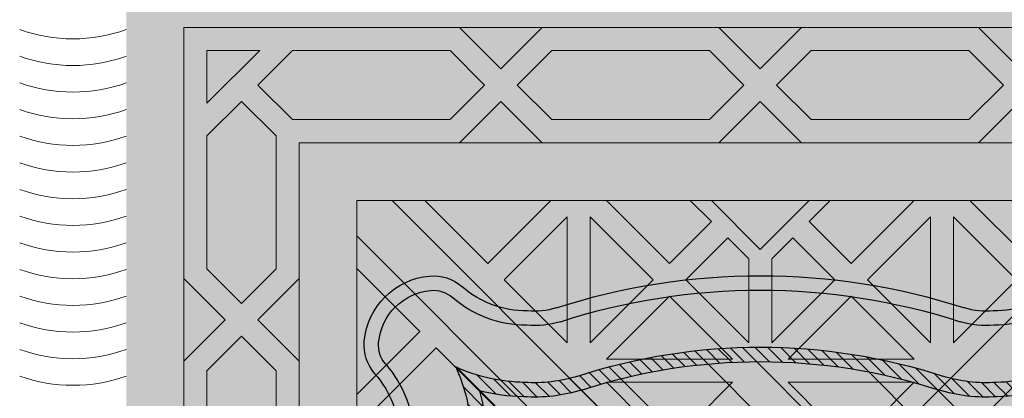
# Model space of a CAD drawing. Units: inches. Extents: x 844 to 2234, y 346 to 1084.
# Tile 33 of 93: x 1249.18 to 1260.07, y 703.6 to 707.78. Entities that reach past the tile are written whole.
import ezdxf

# ---------------------------------------------------------------- set-up
doc = ezdxf.new("R2010")
doc.units = ezdxf.units.IN
doc.header["$MEASUREMENT"] = 0
doc.layers.add('furniture', color=8, linetype='Continuous', lineweight=18)
doc.layers.add('RA-AP-01$0$INT', color=35, linetype='Continuous', lineweight=5)
doc.layers.add('RA-AP-01$0$FURN', color=3, linetype='Continuous')
doc.layers.add('RA-AP-01$0$WOOD', color=64, linetype='Continuous')

# ---------------------------------------------------------------- blocks, each defined once
blk = doc.blocks.new('A$C18D01794')
at = {"layer": 'RA-AP-01$0$INT'}
h = blk.add_hatch(color=256, dxfattribs=at)
h.paths.add_polyline_path([(4.35521, -6.15671), (4.35521, -8.05671), (5.45521, -8.05671), (5.45521, -6.15671)])
h.paths.add_polyline_path([(4.40521, -8.00671), (4.40521, -6.20671), (5.40521, -6.20671), (5.40521, -8.00671)], flags=16)
h = blk.add_hatch(color=256, dxfattribs=at)
h.paths.add_polyline_path([(4.50521, -7.5855), (4.46935, -7.54964), (4.50521, -7.51378), (4.50521, -7.38196), (4.46935, -7.34611), (4.50521, -7.31025), (4.50521, -7.17843), (4.46935, -7.14257), (4.50521, -7.10671), (4.47692, -7.10671), (4.45521, -7.12843), (4.43349, -7.10671), (4.40521, -7.10671), (4.44106, -7.14257), (4.40521, -7.17843), (4.40521, -7.31025), (4.44106, -7.34611), (4.40521, -7.38196), (4.40521, -7.51378), (4.44106, -7.54964), (4.40521, -7.5855), (4.40521, -7.71732), (4.44106, -7.75318), (4.40521, -7.78903), (4.40521, -8.00671), (4.64435, -8.00671), (4.68021, -7.97085), (4.71606, -8.00671), (4.86935, -8.00671), (4.90521, -7.97085), (4.94106, -8.00671), (5.09435, -8.00671), (5.13021, -7.97085), (5.16606, -8.00671), (5.40521, -8.00671), (5.40521, -7.78903), (5.36935, -7.75318), (5.40521, -7.71732), (5.40521, -7.5855), (5.36935, -7.54964), (5.40521, -7.51378), (5.40521, -7.38196), (5.36935, -7.34611), (5.40521, -7.31025), (5.40521, -7.17843), (5.36935, -7.14257), (5.40521, -7.10671), (5.37692, -7.10671), (5.35521, -7.12843), (5.33349, -7.10671), (5.30521, -7.10671), (5.34106, -7.14257), (5.30521, -7.17843), (5.30521, -7.31025), (5.34106, -7.34611), (5.30521, -7.38196), (5.30521, -7.51378), (5.34106, -7.54964), (5.30521, -7.5855), (5.30521, -7.71732), (5.34106, -7.75318), (5.30521, -7.78903), (5.30521, -7.90671), (5.16606, -7.90671), (5.13021, -7.94257), (5.09435, -7.90671), (4.94106, -7.90671), (4.90521, -7.94257), (4.86935, -7.90671), (4.71606, -7.90671), (4.68021, -7.94257), (4.64435, -7.90671), (4.50521, -7.90671), (4.50521, -7.78903), (4.46935, -7.75318), (4.50521, -7.71732)])
h.paths.add_polyline_path([(4.48521, -7.70903), (4.45521, -7.73903), (4.42521, -7.70903), (4.42521, -7.59378), (4.45521, -7.56378), (4.48521, -7.59378)], flags=16)
h.paths.add_polyline_path([(4.45521, -7.76732), (4.48521, -7.79732), (4.48521, -7.91257), (4.45521, -7.94257), (4.42521, -7.91257), (4.42521, -7.79732)], flags=16)
h.paths.add_polyline_path([(4.45521, -7.5355), (4.42521, -7.5055), (4.42521, -7.39025), (4.45521, -7.36025), (4.48521, -7.39025), (4.48521, -7.5055)], flags=16)
h.paths.add_polyline_path([(4.49935, -7.92671), (4.63606, -7.92671), (4.66606, -7.95671), (4.63606, -7.98671), (4.49935, -7.98671), (4.46935, -7.95671)], flags=16)
h.paths.add_polyline_path([(4.42521, -7.94085), (4.47106, -7.98671), (4.42521, -7.98671)], flags=16)
h.paths.add_polyline_path([(4.45521, -7.33196), (4.42521, -7.30196), (4.42521, -7.18671), (4.45521, -7.15671), (4.48521, -7.18671), (4.48521, -7.30196)], flags=16)
h.paths.add_polyline_path([(4.72435, -7.92671), (4.86106, -7.92671), (4.89106, -7.95671), (4.86106, -7.98671), (4.72435, -7.98671), (4.69435, -7.95671)], flags=16)
h.paths.add_polyline_path([(4.91935, -7.95671), (4.94935, -7.92671), (5.08606, -7.92671), (5.11606, -7.95671), (5.08606, -7.98671), (4.94935, -7.98671)], flags=16)
h.paths.add_polyline_path([(5.14435, -7.95671), (5.17435, -7.92671), (5.31106, -7.92671), (5.34106, -7.95671), (5.31106, -7.98671), (5.17435, -7.98671)], flags=16)
h.paths.add_polyline_path([(5.32521, -7.59378), (5.35521, -7.56378), (5.38521, -7.59378), (5.38521, -7.70903), (5.35521, -7.73903), (5.32521, -7.70903)], flags=16)
h.paths.add_polyline_path([(5.32521, -7.79732), (5.35521, -7.76732), (5.38521, -7.79732), (5.38521, -7.91257), (5.35521, -7.94257), (5.32521, -7.91257)], flags=16)
h.paths.add_polyline_path([(5.32521, -7.5055), (5.32521, -7.39025), (5.35521, -7.36025), (5.38521, -7.39025), (5.38521, -7.5055), (5.35521, -7.5355)], flags=16)
h.paths.add_polyline_path([(5.32521, -7.30196), (5.32521, -7.18671), (5.35521, -7.15671), (5.38521, -7.18671), (5.38521, -7.30196), (5.35521, -7.33196)], flags=16)
h.paths.add_polyline_path([(5.33935, -7.98671), (5.38521, -7.94085), (5.38521, -7.98671)], flags=16)
h = blk.add_hatch(color=256, dxfattribs=at)
h.paths.add_polyline_path([(4.46935, -7.14257), (4.50521, -7.17843), (4.50521, -7.10671)])
h.paths.add_polyline_path([(4.45521, -7.12843), (4.47692, -7.10671), (4.43349, -7.10671)])
h.paths.add_polyline_path([(4.40521, -7.17843), (4.44106, -7.14257), (4.40521, -7.10671)])
h.paths.add_polyline_path([(4.42521, -7.30196), (4.45521, -7.33196), (4.48521, -7.30196), (4.48521, -7.18671), (4.45521, -7.15671), (4.42521, -7.18671)])
h.paths.add_polyline_path([(4.50521, -7.38196), (4.50521, -7.31025), (4.46935, -7.34611)])
h.paths.add_polyline_path([(4.42521, -7.5055), (4.45521, -7.5355), (4.48521, -7.5055), (4.48521, -7.39025), (4.45521, -7.36025), (4.42521, -7.39025)])
h.paths.add_polyline_path([(4.42521, -7.70903), (4.45521, -7.73903), (4.48521, -7.70903), (4.48521, -7.59378), (4.45521, -7.56378), (4.42521, -7.59378)])
h.paths.add_polyline_path([(4.46935, -7.54964), (4.50521, -7.5855), (4.50521, -7.51378)])
h.paths.add_polyline_path([(4.40521, -7.5855), (4.44106, -7.54964), (4.40521, -7.51378)])
h.paths.add_polyline_path([(4.40521, -7.78903), (4.44106, -7.75318), (4.40521, -7.71732)])
h.paths.add_polyline_path([(4.46935, -7.75318), (4.50521, -7.78903), (4.50521, -7.71732)])
h.paths.add_polyline_path([(4.42521, -7.91257), (4.45521, -7.94257), (4.48521, -7.91257), (4.48521, -7.79732), (4.45521, -7.76732), (4.42521, -7.79732)])
h.paths.add_polyline_path([(4.42521, -7.98671), (4.47106, -7.98671), (4.42521, -7.94085)])
h.paths.add_polyline_path([(4.49935, -7.98671), (4.63606, -7.98671), (4.66606, -7.95671), (4.63606, -7.92671), (4.49935, -7.92671), (4.46935, -7.95671)])
h.paths.add_polyline_path([(4.68021, -7.94257), (4.71606, -7.90671), (4.64435, -7.90671)])
h.paths.add_polyline_path([(4.64435, -8.00671), (4.71606, -8.00671), (4.68021, -7.97085)])
h.paths.add_polyline_path([(4.72435, -7.98671), (4.86106, -7.98671), (4.89106, -7.95671), (4.86106, -7.92671), (4.72435, -7.92671), (4.69435, -7.95671)])
h.paths.add_polyline_path([(4.90521, -7.94257), (4.94106, -7.90671), (4.86935, -7.90671)])
h.paths.add_polyline_path([(4.86935, -8.00671), (4.94106, -8.00671), (4.90521, -7.97085)])
h.paths.add_polyline_path([(4.94935, -7.98671), (5.08606, -7.98671), (5.11606, -7.95671), (5.08606, -7.92671), (4.94935, -7.92671), (4.91935, -7.95671)])
h.paths.add_polyline_path([(5.13021, -7.94257), (5.16606, -7.90671), (5.09435, -7.90671)])
h.paths.add_polyline_path([(5.09435, -8.00671), (5.16606, -8.00671), (5.13021, -7.97085)])
h.paths.add_polyline_path([(5.17435, -7.98671), (5.31106, -7.98671), (5.34106, -7.95671), (5.31106, -7.92671), (5.17435, -7.92671), (5.14435, -7.95671)])
h.paths.add_polyline_path([(5.32521, -7.91257), (5.35521, -7.94257), (5.38521, -7.91257), (5.38521, -7.79732), (5.35521, -7.76732), (5.32521, -7.79732)])
h.paths.add_polyline_path([(5.33935, -7.98671), (5.38521, -7.98671), (5.38521, -7.94085)])
h.paths.add_polyline_path([(5.32521, -7.70903), (5.35521, -7.73903), (5.38521, -7.70903), (5.38521, -7.59378), (5.35521, -7.56378), (5.32521, -7.59378)])
h.paths.add_polyline_path([(5.30521, -7.78903), (5.34106, -7.75318), (5.30521, -7.71732)])
h.paths.add_polyline_path([(5.36935, -7.75318), (5.40521, -7.78903), (5.40521, -7.71732)])
h.paths.add_polyline_path([(5.40521, -7.5855), (5.40521, -7.51378), (5.36935, -7.54964)])
h.paths.add_polyline_path([(5.30521, -7.5855), (5.34106, -7.54964), (5.30521, -7.51378)])
h.paths.add_polyline_path([(5.32521, -7.5055), (5.35521, -7.5355), (5.38521, -7.5055), (5.38521, -7.39025), (5.35521, -7.36025), (5.32521, -7.39025)])
h.paths.add_polyline_path([(5.30521, -7.38196), (5.34106, -7.34611), (5.30521, -7.31025)])
h.paths.add_polyline_path([(5.32521, -7.30196), (5.35521, -7.33196), (5.38521, -7.30196), (5.38521, -7.18671), (5.35521, -7.15671), (5.32521, -7.18671)])
h.paths.add_polyline_path([(5.40458, -7.38134, -0.001218), (5.40521, -7.38111), (5.40521, -7.31025), (5.36935, -7.34611)])
h.paths.add_polyline_path([(5.36935, -7.14257), (5.40521, -7.17843), (5.40521, -7.10671)])
h.paths.add_polyline_path([(5.35521, -7.12843), (5.37692, -7.10671), (5.33349, -7.10671)])
h.paths.add_polyline_path([(5.30521, -7.17843), (5.34106, -7.14257), (5.30521, -7.10671)])
blk.add_hatch(color=256, dxfattribs=at).paths.add_polyline_path([(4.50521, -7.90671), (5.30521, -7.90671), (5.30521, -7.10671), (5.25521, -7.10671), (5.25521, -7.85671), (4.55521, -7.85671), (4.55521, -7.10671), (4.50521, -7.10671)])
h = blk.add_hatch(color=256, dxfattribs=at)
h.paths.add_polyline_path([(4.58592, -7.85671), (4.6142, -7.85671), (4.66885, -7.80207), (4.72349, -7.85671), (4.77177, -7.85671), (4.82642, -7.80207), (4.86278, -7.83843), (4.8445, -7.85671), (4.86278, -7.85671), (4.90521, -7.81429), (4.94763, -7.85671), (4.96592, -7.85671), (4.94763, -7.83843), (4.98399, -7.80207), (5.03864, -7.85671), (5.08692, -7.85671), (5.14157, -7.80207), (5.19621, -7.85671), (5.2245, -7.85671), (4.90521, -7.53742)])
h.paths.add_polyline_path([(4.89521, -7.57571), (4.89521, -7.685), (4.84056, -7.63035)], flags=16)
h.paths.add_polyline_path([(4.91521, -7.57571), (4.96985, -7.63035), (4.91521, -7.685)], flags=16)
h.paths.add_polyline_path([(4.82642, -7.64449), (4.88106, -7.69914), (4.77177, -7.69914)], flags=16)
h.paths.add_polyline_path([(4.98399, -7.64449), (5.03864, -7.69914), (4.92935, -7.69914)], flags=16)
h.paths.add_polyline_path([(4.88106, -7.71914), (4.82642, -7.77378), (4.77177, -7.71914)], flags=16)
h.paths.add_polyline_path([(4.92935, -7.71914), (5.03864, -7.71914), (4.98399, -7.77378)], flags=16)
h.paths.add_polyline_path([(4.89521, -7.73328), (4.89521, -7.806), (4.87692, -7.82429), (4.84056, -7.78793)], flags=16)
h.paths.add_polyline_path([(4.91521, -7.73328), (4.96985, -7.78793), (4.93349, -7.82429), (4.91521, -7.806)], flags=16)
h.paths.add_polyline_path([(4.75763, -7.73328), (4.81228, -7.78793), (4.75763, -7.84257)], flags=16)
h.paths.add_polyline_path([(4.73763, -7.73328), (4.73763, -7.84257), (4.68299, -7.78793)], flags=16)
h.paths.add_polyline_path([(5.05278, -7.73328), (5.05278, -7.84257), (4.99814, -7.78793)], flags=16)
h.paths.add_polyline_path([(5.07278, -7.73328), (5.12742, -7.78793), (5.07278, -7.84257)], flags=16)
h.paths.add_polyline_path([(4.93592, -7.50671), (5.25521, -7.826), (5.25521, -7.79772), (5.20056, -7.74307), (5.25521, -7.68843), (5.25521, -7.64014), (5.20056, -7.5855), (5.23692, -7.54914), (5.25521, -7.56742), (5.25521, -7.54914), (5.21278, -7.50671), (5.25521, -7.46429), (5.25521, -7.446), (5.23692, -7.46429), (5.20056, -7.42793), (5.25521, -7.37328), (5.25521, -7.325), (5.20056, -7.27035), (5.25521, -7.21571), (5.25521, -7.18742)])
h.paths.add_polyline_path([(5.04299, -7.42793), (5.09763, -7.37328), (5.09763, -7.48257)], flags=16)
h.paths.add_polyline_path([(5.02885, -7.44207), (5.08349, -7.49671), (4.9742, -7.49671)], flags=16)
h.paths.add_polyline_path([(5.11763, -7.37328), (5.17228, -7.42793), (5.11763, -7.48257)], flags=16)
h.paths.add_polyline_path([(5.08349, -7.51671), (5.02885, -7.57136), (4.9742, -7.51671)], flags=16)
h.paths.add_polyline_path([(5.13177, -7.35914), (5.18642, -7.41378), (5.24106, -7.35914)], flags=17)
h.paths.add_polyline_path([(5.13177, -7.49671), (5.18642, -7.44207), (5.22278, -7.47843), (5.2045, -7.49671)], flags=16)
h.paths.add_polyline_path([(5.09763, -7.53085), (5.09763, -7.64014), (5.04299, -7.5855)], flags=16)
h.paths.add_polyline_path([(5.13177, -7.33914), (5.24106, -7.33914), (5.18642, -7.28449)], flags=17)
h.paths.add_polyline_path([(5.13177, -7.51671), (5.2045, -7.51671), (5.22278, -7.535), (5.18642, -7.57136)], flags=16)
h.paths.add_polyline_path([(5.11763, -7.53085), (5.17228, -7.5855), (5.11763, -7.64014)], flags=16)
h.paths.add_polyline_path([(5.18642, -7.59964), (5.24106, -7.65429), (5.13177, -7.65429)], flags=16)
h.paths.add_polyline_path([(5.13177, -7.67429), (5.24106, -7.67429), (5.18642, -7.72893)], flags=16)
h.paths.add_polyline_path([(5.25521, -7.126), (5.25521, -7.10671), (4.55521, -7.10671), (4.55521, -7.126), (4.90521, -7.476)])
h.paths.add_polyline_path([(4.98399, -7.36893), (4.92935, -7.31429), (5.03864, -7.31429)], flags=16)
h.paths.add_polyline_path([(4.96985, -7.38307), (4.91521, -7.43772), (4.91521, -7.32843)], flags=16)
h.paths.add_polyline_path([(4.92935, -7.29429), (4.98399, -7.23964), (5.03864, -7.29429)], flags=16)
h.paths.add_polyline_path([(5.05278, -7.28014), (4.99814, -7.2255), (5.05278, -7.17085)], flags=16)
h.paths.add_polyline_path([(5.07278, -7.28014), (5.07278, -7.17085), (5.12742, -7.2255)], flags=16)
h.paths.add_polyline_path([(4.89521, -7.43772), (4.84056, -7.38307), (4.89521, -7.32843)], flags=16)
h.paths.add_polyline_path([(4.91521, -7.28014), (4.91521, -7.20742), (4.93349, -7.18914), (4.96985, -7.2255)], flags=16)
h.paths.add_polyline_path([(4.88106, -7.31429), (4.82642, -7.36893), (4.77177, -7.31429)], flags=16)
h.paths.add_polyline_path([(4.89521, -7.28014), (4.84056, -7.2255), (4.87692, -7.18914), (4.89521, -7.20742)], flags=16)
h.paths.add_polyline_path([(4.98399, -7.21136), (4.94763, -7.175), (4.96592, -7.15671), (5.03864, -7.15671)], flags=16)
h.paths.add_polyline_path([(4.88106, -7.29429), (4.77177, -7.29429), (4.82642, -7.23964)], flags=16)
h.paths.add_polyline_path([(4.90521, -7.19914), (4.86278, -7.15671), (4.94763, -7.15671)], flags=16)
h.paths.add_polyline_path([(5.14157, -7.21136), (5.08692, -7.15671), (5.19621, -7.15671)], flags=16)
h.paths.add_polyline_path([(4.82642, -7.21136), (4.77177, -7.15671), (4.8445, -7.15671), (4.86278, -7.175)], flags=16)
h.paths.add_polyline_path([(4.81228, -7.2255), (4.75763, -7.28014), (4.75763, -7.17085)], flags=16)
h.paths.add_polyline_path([(4.73763, -7.28014), (4.68299, -7.2255), (4.73763, -7.17085)], flags=16)
h.paths.add_polyline_path([(4.72349, -7.15671), (4.66885, -7.21136), (4.6142, -7.15671)], flags=16)
h.paths.add_polyline_path([(4.59763, -7.50671), (4.55521, -7.54914), (4.55521, -7.56742), (4.57349, -7.54914), (4.60985, -7.5855), (4.55521, -7.64014), (4.55521, -7.68843), (4.60985, -7.74307), (4.55521, -7.79772), (4.55521, -7.826), (4.8745, -7.50671), (4.55521, -7.18742), (4.55521, -7.21571), (4.60985, -7.27035), (4.55521, -7.325), (4.55521, -7.37328), (4.60985, -7.42793), (4.57349, -7.46429), (4.55521, -7.446), (4.55521, -7.46429)])
h.paths.add_polyline_path([(4.71278, -7.48257), (4.71278, -7.37328), (4.76742, -7.42793)], flags=16)
h.paths.add_polyline_path([(4.72692, -7.49671), (4.78157, -7.44207), (4.83621, -7.49671)], flags=16)
h.paths.add_polyline_path([(4.69278, -7.48257), (4.63814, -7.42793), (4.69278, -7.37328)], flags=16)
h.paths.add_polyline_path([(4.72692, -7.51671), (4.83621, -7.51671), (4.78157, -7.57136)], flags=16)
h.paths.add_polyline_path([(4.67864, -7.49671), (4.60592, -7.49671), (4.58763, -7.47843), (4.62399, -7.44207)], flags=16)
h.paths.add_polyline_path([(4.71278, -7.53085), (4.76742, -7.5855), (4.71278, -7.64014)], flags=16)
h.paths.add_polyline_path([(4.67864, -7.51671), (4.62399, -7.57136), (4.58763, -7.535), (4.60592, -7.51671)], flags=16)
h.paths.add_polyline_path([(4.69278, -7.53085), (4.69278, -7.64014), (4.63814, -7.5855)], flags=16)
h.paths.add_polyline_path([(4.62399, -7.41378), (4.67864, -7.35914), (4.56935, -7.35914)], flags=17)
h.paths.add_polyline_path([(4.62399, -7.59964), (4.67864, -7.65429), (4.56935, -7.65429)], flags=16)
h.paths.add_polyline_path([(4.67864, -7.33914), (4.62399, -7.28449), (4.56935, -7.33914)], flags=17)
h.paths.add_polyline_path([(4.67864, -7.67429), (4.62399, -7.72893), (4.56935, -7.67429)], flags=16)
h = blk.add_hatch(color=256, dxfattribs=at)
h.paths.add_polyline_path([(4.90521, -7.53742), (4.8745, -7.50671), (4.55521, -7.826), (4.55521, -7.85671), (4.58592, -7.85671)])
h.paths.add_polyline_path([(4.93592, -7.50671), (4.90521, -7.53742), (5.2245, -7.85671), (5.25521, -7.85671), (5.25521, -7.826)])
h.paths.add_polyline_path([(5.25521, -7.18742), (5.25521, -7.126), (4.90521, -7.476), (4.93592, -7.50671)])
h.paths.add_polyline_path([(4.8745, -7.50671), (4.90521, -7.476), (4.55521, -7.126), (4.55521, -7.18742)])
h = blk.add_hatch(color=256, dxfattribs=at)
h.paths.add_polyline_path([(5.02885, -7.57136), (4.9742, -7.51671), (5.08349, -7.51671)])
h.paths.add_polyline_path([(4.9742, -7.49671), (5.02885, -7.44207), (5.08349, -7.49671)])
h.paths.add_polyline_path([(5.04299, -7.42793), (5.09763, -7.37328), (5.09763, -7.48257)])
h.paths.add_polyline_path([(5.11763, -7.48257), (5.11763, -7.37328), (5.17228, -7.42793)])
h.paths.add_polyline_path([(5.13177, -7.49671), (5.18642, -7.44207), (5.22278, -7.47843), (5.2045, -7.49671)])
h.paths.add_polyline_path([(5.23692, -7.46429), (5.20056, -7.42793), (5.25521, -7.37328), (5.25521, -7.446)])
h.paths.add_polyline_path([(5.18642, -7.41378), (5.13177, -7.35914), (5.24106, -7.35914)])
h.paths.add_polyline_path([(5.13177, -7.33914), (5.18642, -7.28449), (5.24106, -7.33914)])
h.paths.add_polyline_path([(5.20056, -7.27035), (5.25521, -7.21571), (5.25521, -7.325)])
h.paths.add_polyline_path([(5.21278, -7.50671), (5.25521, -7.46429), (5.25521, -7.54914)])
h.paths.add_polyline_path([(5.13177, -7.51671), (5.2045, -7.51671), (5.22278, -7.535), (5.18642, -7.57136)])
h.paths.add_polyline_path([(5.11763, -7.64014), (5.11763, -7.53085), (5.17228, -7.5855)])
h.paths.add_polyline_path([(5.04299, -7.5855), (5.09763, -7.53085), (5.09763, -7.64014)])
h.paths.add_polyline_path([(5.13177, -7.65429), (5.18642, -7.59964), (5.24106, -7.65429)])
h.paths.add_polyline_path([(5.20056, -7.5855), (5.23692, -7.54914), (5.25521, -7.56742), (5.25521, -7.64014)])
h.paths.add_polyline_path([(5.18642, -7.72893), (5.13177, -7.67429), (5.24106, -7.67429)])
h.paths.add_polyline_path([(5.20056, -7.74307), (5.25521, -7.68843), (5.25521, -7.79772)])
h = blk.add_hatch(color=256, dxfattribs=at)
h.paths.add_polyline_path([(4.96985, -7.63035), (4.91521, -7.57571), (4.91521, -7.685)])
h.paths.add_polyline_path([(4.89521, -7.57571), (4.84056, -7.63035), (4.89521, -7.685)])
h.paths.add_polyline_path([(4.82642, -7.64449), (4.77177, -7.69914), (4.88106, -7.69914)])
h.paths.add_polyline_path([(4.88106, -7.71914), (4.77177, -7.71914), (4.82642, -7.77378)])
h.paths.add_polyline_path([(4.89521, -7.73328), (4.84056, -7.78793), (4.87692, -7.82429), (4.89521, -7.806)])
h.paths.add_polyline_path([(4.86278, -7.83843), (4.82642, -7.80207), (4.77177, -7.85671), (4.8445, -7.85671)])
h.paths.add_polyline_path([(4.81228, -7.78793), (4.75763, -7.73328), (4.75763, -7.84257)])
h.paths.add_polyline_path([(4.73763, -7.73328), (4.68299, -7.78793), (4.73763, -7.84257)])
h.paths.add_polyline_path([(4.66885, -7.80207), (4.6142, -7.85671), (4.72349, -7.85671)])
h.paths.add_polyline_path([(4.90521, -7.81429), (4.86278, -7.85671), (4.94763, -7.85671)])
h.paths.add_polyline_path([(4.91521, -7.73328), (4.91521, -7.806), (4.93349, -7.82429), (4.96985, -7.78793)])
h.paths.add_polyline_path([(5.03864, -7.71914), (4.92935, -7.71914), (4.98399, -7.77378)])
h.paths.add_polyline_path([(4.98399, -7.64449), (4.92935, -7.69914), (5.03864, -7.69914)])
h.paths.add_polyline_path([(5.05278, -7.73328), (4.99814, -7.78793), (5.05278, -7.84257)])
h.paths.add_polyline_path([(4.98399, -7.80207), (4.94763, -7.83843), (4.96592, -7.85671), (5.03864, -7.85671)])
h.paths.add_polyline_path([(5.12742, -7.78793), (5.07278, -7.73328), (5.07278, -7.84257)])
h.paths.add_polyline_path([(5.14157, -7.80207), (5.08692, -7.85671), (5.19621, -7.85671)])
for p, q in [((5.25521, -7.10671), (5.25521, -7.85671)), ((4.8745, -7.50671), (4.55521, -7.826)), ((4.93592, -7.50671), (5.25521, -7.826)), ((4.90521, -7.53742), (4.58592, -7.85671)), ((4.90521, -7.53742), (5.2245, -7.85671)), ((5.32521, -7.59378), (5.32521, -7.70903)), ((5.38521, -7.59378), (5.38521, -7.70903)), ((4.82642, -7.64449), (4.77177, -7.69914)), ((4.88106, -7.69914), (4.82642, -7.64449)), ((4.92935, -7.69914), (4.98399, -7.64449)), ((4.98399, -7.64449), (5.03864, -7.69914)), ((5.18642, -7.72893), (5.13177, -7.67429)), ((5.24106, -7.67429), (5.18642, -7.72893)), ((5.25521, -7.68843), (5.20056, -7.74307)), ((4.77177, -7.69914), (4.88106, -7.69914)), ((5.03864, -7.69914), (4.92935, -7.69914)), ((5.32521, -7.70903), (5.35521, -7.73903)), ((5.38521, -7.70903), (5.35521, -7.73903)), ((4.77177, -7.71914), (4.88106, -7.71914)), ((4.77177, -7.71914), (4.82642, -7.77378)), ((4.88106, -7.71914), (4.82642, -7.77378)), ((5.03864, -7.71914), (4.92935, -7.71914)), ((4.92935, -7.71914), (4.98399, -7.77378)), ((5.03864, -7.71914), (4.98399, -7.77378)), ((5.30521, -7.71732), (5.34106, -7.75318)), ((5.40521, -7.71732), (5.36935, -7.75318)), ((4.68299, -7.78793), (4.73763, -7.73328)), ((4.73763, -7.73328), (4.73763, -7.84257)), ((4.75763, -7.73328), (4.81228, -7.78793)), ((4.75763, -7.73328), (4.75763, -7.84257)), ((4.89521, -7.73328), (4.84056, -7.78793)), ((4.89521, -7.806), (4.89521, -7.73328)), ((4.91521, -7.806), (4.91521, -7.73328)), ((4.91521, -7.73328), (4.96985, -7.78793)), ((5.05278, -7.73328), (4.99814, -7.78793)), ((5.05278, -7.73328), (5.05278, -7.84257)), ((5.12742, -7.78793), (5.07278, -7.73328)), ((5.07278, -7.73328), (5.07278, -7.84257)), ((5.25521, -7.79772), (5.20056, -7.74307)), ((5.34106, -7.75318), (5.30521, -7.78903)), ((5.36935, -7.75318), (5.40521, -7.78903)), ((5.35521, -7.76732), (5.32521, -7.79732)), ((5.35521, -7.76732), (5.38521, -7.79732)), ((4.73763, -7.84257), (4.68299, -7.78793)), ((4.75763, -7.84257), (4.81228, -7.78793)), ((4.84056, -7.78793), (4.87692, -7.82429)), ((4.96985, -7.78793), (4.93349, -7.82429)), ((5.05278, -7.84257), (4.99814, -7.78793)), ((5.07278, -7.84257), (5.12742, -7.78793)), ((5.32521, -7.91257), (5.32521, -7.79732)), ((5.38521, -7.79732), (5.38521, -7.91257)), ((4.72349, -7.85671), (4.66885, -7.80207)), ((4.77177, -7.85671), (4.82642, -7.80207)), ((4.82642, -7.80207), (4.86278, -7.83843)), ((4.98399, -7.80207), (4.94763, -7.83843)), ((5.03864, -7.85671), (4.98399, -7.80207)), ((5.08692, -7.85671), (5.14157, -7.80207)), ((5.19621, -7.85671), (5.14157, -7.80207)), ((4.90521, -7.81429), (4.86278, -7.85671)), ((4.89521, -7.806), (4.87692, -7.82429)), ((4.90521, -7.81429), (4.94763, -7.85671)), ((4.91521, -7.806), (4.93349, -7.82429)), ((4.8445, -7.85671), (4.86278, -7.83843)), ((4.94763, -7.83843), (4.96592, -7.85671)), ((4.96592, -7.85671), (4.94763, -7.83843)), ((4.55521, -7.85671), (5.25521, -7.85671)), ((4.8445, -7.85671), (4.77177, -7.85671)), ((4.94763, -7.85671), (4.86278, -7.85671)), ((4.96592, -7.85671), (5.03864, -7.85671)), ((5.26721, -7.90671), (4.54321, -7.90671)), ((5.26721, -7.90671), (4.54321, -7.90671)), ((4.71606, -7.90671), (4.68021, -7.94257)), ((4.86935, -7.90671), (4.90521, -7.94257)), ((4.94106, -7.90671), (4.90521, -7.94257)), ((5.09435, -7.90671), (5.13021, -7.94257)), ((5.16606, -7.90671), (5.13021, -7.94257)), ((5.32521, -7.91257), (5.35521, -7.94257)), ((5.38521, -7.91257), (5.35521, -7.94257)), ((4.72435, -7.92671), (4.69435, -7.95671)), ((4.86106, -7.92671), (4.72435, -7.92671)), ((4.86106, -7.92671), (4.89106, -7.95671)), ((4.94935, -7.92671), (4.91935, -7.95671)), ((4.94935, -7.92671), (5.08606, -7.92671)), ((5.08606, -7.92671), (5.11606, -7.95671)), ((5.17435, -7.92671), (5.14435, -7.95671)), ((5.17435, -7.92671), (5.31106, -7.92671)), ((5.31106, -7.92671), (5.34106, -7.95671)), ((5.33935, -7.98671), (5.38521, -7.94085)), ((5.38521, -7.94085), (5.38521, -7.98671)), ((4.72435, -7.98671), (4.69435, -7.95671)), ((4.86106, -7.98671), (4.89106, -7.95671)), ((4.94935, -7.98671), (4.91935, -7.95671)), ((5.08606, -7.98671), (5.11606, -7.95671)), ((5.17435, -7.98671), (5.14435, -7.95671)), ((5.31106, -7.98671), (5.34106, -7.95671)), ((4.71606, -8.00671), (4.68021, -7.97085)), ((4.86935, -8.00671), (4.90521, -7.97085)), ((4.94106, -8.00671), (4.90521, -7.97085)), ((5.09435, -8.00671), (5.13021, -7.97085)), ((5.16606, -8.00671), (5.13021, -7.97085)), ((4.86106, -7.98671), (4.72435, -7.98671)), ((4.94935, -7.98671), (5.08606, -7.98671)), ((5.17435, -7.98671), (5.31106, -7.98671)), ((5.33935, -7.98671), (5.38521, -7.98671))]:
    blk.add_line(p, q, dxfattribs=at)
for points in [[(5.40521, -8.00671), (4.40521, -8.00671), (4.40521, -7.10671)], [(5.30521, -7.10671), (5.30521, -7.90671), (4.50521, -7.90671), (4.50521, -7.10671)], [(5.40521, -7.10671), (5.40521, -8.00671)]]:
    blk.add_lwpolyline(points, dxfattribs=at)
for centre in [(5.50141, -7.83286), (5.50141, -7.85596), (5.50141, -7.87906), (5.50141, -7.90216), (5.50141, -7.92526), (5.50141, -7.94836), (5.50141, -7.97146), (5.50141, -7.99456), (5.50141, -8.01766), (5.50141, -8.04076), (5.50141, -8.06386), (5.50141, -8.08696), (5.50141, -8.11006), (5.50141, -8.13316)]:
    blk.add_arc(centre, 0.13641, 70.20384, 109.79616, dxfattribs=at)
blk = doc.blocks.new('A$C32926AE1')
at = {"layer": 'RA-AP-01$0$WOOD'}
h = blk.add_hatch(color=256, dxfattribs=at)
h.dxf.hatch_style = 1
h.paths.add_polyline_path([(5.15743, 4.57348, -0.100949), (5.1554, 4.59337, -0.184266), (5.17225, 4.6388, 0.205661), (5.17956, 4.66132, 0.361434), (5.13435, 4.70652, 0.205661), (5.11183, 4.69921, -0.184266), (5.0664, 4.68237, -0.105531), (5.04566, 4.68467, 0.156764), (4.76389, 4.68467, -0.105531), (4.74314, 4.68237, -0.184266), (4.69771, 4.69921, 0.205661), (4.67519, 4.70652, 0.361434), (4.62998, 4.66132, 0.205661), (4.63729, 4.6388, -0.184266), (4.65414, 4.59337, -0.100949), (4.65211, 4.57348, 0.02141), (4.62975, 4.15671, 0.02141), (4.65211, 3.73994, -0.100949), (4.65414, 3.72006, -0.184266), (4.63729, 3.67463, 0.205661), (4.62998, 3.65211, 0.361434), (4.67519, 3.6069, 0.205661), (4.69771, 3.61421, -0.184266), (4.74314, 3.63106, -0.105531), (4.76389, 3.62875, 0.156764), (5.04566, 3.62875, -0.105531), (5.0664, 3.63106, -0.184266), (5.11183, 3.61421, 0.205661), (5.13435, 3.6069, 0.361434), (5.17956, 3.65211, 0.205661), (5.17225, 3.67463, -0.184266), (5.1554, 3.72006, -0.100949), (5.15743, 3.73994, 0.02141), (5.17979, 4.15671, 0.02141)])
h.paths.add_polyline_path([(4.63975, 4.15671, 0.021354), (4.66197, 3.74189, -0.094076), (4.66414, 3.71961, -0.182482), (4.64481, 3.66804, 0.205661), (4.63994, 3.65302, 0.361434), (4.67611, 3.61686, 0.205661), (4.69112, 3.62173, -0.182482), (4.7427, 3.64106, -0.102989), (4.76699, 3.63826, 0.156709), (5.04255, 3.63826, -0.102989), (5.06685, 3.64106, -0.182482), (5.11842, 3.62173, 0.205661), (5.13344, 3.61686, 0.361434), (5.1696, 3.65302, 0.205661), (5.16473, 3.66804, -0.182482), (5.1454, 3.71961, -0.094076), (5.14757, 3.74189, 0.021354), (5.16979, 4.15671, 0.021354), (5.14757, 4.57154, -0.094076), (5.1454, 4.59381, -0.182482), (5.16473, 4.64539, 0.205661), (5.1696, 4.6604, 0.361434), (5.13344, 4.69657, 0.205661), (5.11842, 4.69169, -0.182482), (5.06685, 4.67236, -0.102989), (5.04255, 4.67517, 0.156709), (4.76699, 4.67517, -0.102989), (4.7427, 4.67236, -0.182482), (4.69112, 4.69169, 0.205661), (4.67611, 4.69657, 0.361434), (4.63994, 4.6604, 0.205661), (4.64481, 4.64539, -0.182482), (4.66414, 4.59381, -0.094076), (4.66197, 4.57154, 0.021354)], flags=16)
h.paths.add_polyline_path([(5.12979, 4.43217, -0.014166), (5.13015, 4.15693, -0.014166), (5.12979, 3.88169, -0.078525), (5.1098, 3.75514, 0.094597), (5.10541, 3.7179, 0.104317), (5.11607, 3.67039, 0.104317), (5.06856, 3.68105, 0.094597), (5.03132, 3.67666, -0.158024), (4.77823, 3.67666, 0.094597), (4.74098, 3.68105, 0.104317), (4.69347, 3.67039, 0.104317), (4.70413, 3.7179, 0.094597), (4.69975, 3.75514, -0.078525), (4.67975, 3.88169, -0.014166), (4.67939, 4.15693, -0.014166), (4.67975, 4.43217, -0.078525), (4.69975, 4.55871, 0.094597), (4.70413, 4.59596, 0.104317), (4.69347, 4.64347, 0.104317), (4.74098, 4.6328, 0.094597), (4.77823, 4.63719, -0.158024), (5.03132, 4.63719, 0.094597), (5.06856, 4.6328, 0.104317), (5.11607, 4.64347, 0.104317), (5.10541, 4.59596, 0.094597), (5.1098, 4.55871, -0.078525)], flags=0)
h.paths.add_polyline_path([(5.11979, 4.43226, -0.0142), (5.12016, 4.15693, -0.0142), (5.11979, 3.8816, -0.078489), (5.10027, 3.75819, 0.094014), (5.09541, 3.71748, 0.060627), (5.09962, 3.68684, 0.060627), (5.06898, 3.69105, 0.094014), (5.02827, 3.68619, -0.158071), (4.78127, 3.68619, 0.094014), (4.74056, 3.69105, 0.060627), (4.70993, 3.68684, 0.060627), (4.71413, 3.71748, 0.094014), (4.70927, 3.75819, -0.078489), (4.68975, 3.8816, -0.0142), (4.68939, 4.15693, -0.0142), (4.68975, 4.43226, -0.078489), (4.70927, 4.55566, 0.094014), (4.71413, 4.59638, 0.060627), (4.70993, 4.62701, 0.060627), (4.74056, 4.62281, 0.094014), (4.78127, 4.62767, -0.158071), (5.02827, 4.62767, 0.094014), (5.06898, 4.62281, 0.060627), (5.09962, 4.62701, 0.060627), (5.09541, 4.59638, 0.094014), (5.10027, 4.55566, -0.078489)], flags=0)
h.paths.add_polyline_path([(5.06979, 4.43022, -0.014242), (5.07017, 4.15693, -0.014242), (5.06979, 3.88364, -0.080061), (5.05266, 3.77346, 0.052642), (5.04591, 3.74055, 0.052642), (5.013, 3.7338, -0.158303), (4.79655, 3.7338, 0.052642), (4.76363, 3.74055, 0.052642), (4.75688, 3.77346, -0.080061), (4.73975, 3.88364, -0.014242), (4.73937, 4.15693, -0.014242), (4.73975, 4.43022, -0.080061), (4.75688, 4.54039, 0.052642), (4.76363, 4.5733, 0.052642), (4.79655, 4.58006, -0.158303), (5.013, 4.58006, 0.052642), (5.04591, 4.5733, 0.052642), (5.05266, 4.54039, -0.080061)], flags=0)
h.paths.add_polyline_path([(5.04979, 4.43038, -0.01431), (5.05018, 4.15693, -0.01431), (5.04979, 3.88347, -0.080069), (5.03362, 3.77958, 0.030626), (5.02824, 3.75822, 0.030626), (5.00688, 3.75284, -0.158398), (4.80266, 3.75284, 0.030626), (4.7813, 3.75822, 0.030626), (4.77592, 3.77958, -0.080069), (4.75975, 3.88347, -0.01431), (4.75936, 4.15693, -0.01431), (4.75975, 4.43038, -0.080069), (4.77592, 4.53427, 0.030626), (4.7813, 4.55564, 0.030626), (4.80266, 4.56102, -0.158398), (5.00688, 4.56102, 0.030626), (5.02824, 4.55564, 0.030626), (5.03362, 4.53427, -0.080069)], flags=0)
h.paths.add_polyline_path([(4.99977, 4.42817, -0.014344), (5.0002, 4.15693, -0.014344), (4.99977, 3.88568, -0.078464), (4.98736, 3.7991, -0.150605), (4.82219, 3.7991, -0.078464), (4.80978, 3.88568, -0.014344), (4.80934, 4.15693, -0.014344), (4.80978, 4.42817, -0.078464), (4.82219, 4.51475, -0.150605), (4.98736, 4.51475, -0.078464)], flags=0)
h.paths.add_polyline_path([(4.97976, 4.42764, -0.014377), (4.98021, 4.15693, -0.014377), (4.97976, 3.88621, -0.068924), (4.97118, 3.81528, -0.129665), (4.83836, 3.81528, -0.068924), (4.82979, 3.88621, -0.014377), (4.82934, 4.15693, -0.014377), (4.82979, 4.42764, -0.068924), (4.83836, 4.49858, -0.129665), (4.97118, 4.49858, -0.068924)], flags=0)
h = blk.add_hatch(color=256, dxfattribs=at)
h.dxf.hatch_style = 1
h.paths.add_polyline_path([(5.1454, 4.59381, -0.182482), (5.16473, 4.64539, 0.205661), (5.1696, 4.6604, 0.361434), (5.13344, 4.69657, 0.205661), (5.11842, 4.69169, -0.182482), (5.06685, 4.67236, -0.102989), (5.04255, 4.67517, 0.156709), (4.76699, 4.67517, -0.102989), (4.7427, 4.67236, -0.182482), (4.69112, 4.69169, 0.205661), (4.67611, 4.69657, 0.361434), (4.63994, 4.6604, 0.205661), (4.64481, 4.64539, -0.182482), (4.66414, 4.59381, -0.094076), (4.66197, 4.57154, 0.021354), (4.63975, 4.15671, 0.021354), (4.66197, 3.74189, -0.094076), (4.66414, 3.71961, -0.182482), (4.64481, 3.66804, 0.205661), (4.63994, 3.65302, 0.361434), (4.67611, 3.61686, 0.205661), (4.69112, 3.62173, -0.182482), (4.7427, 3.64106, -0.102989), (4.76699, 3.63826, 0.156709), (5.04255, 3.63826, -0.102989), (5.06685, 3.64106, -0.182482), (5.11842, 3.62173, 0.205661), (5.13344, 3.61686, 0.361434), (5.1696, 3.65302, 0.205661), (5.16473, 3.66804, -0.182482), (5.1454, 3.71961, -0.094076), (5.14757, 3.74189, 0.021354), (5.16979, 4.15671, 0.021354), (5.14757, 4.57154, -0.094076)])
h.paths.add_polyline_path([(5.1098, 4.55871, -0.078525), (5.12979, 4.43217, -0.014166), (5.13015, 4.15693, -0.014166), (5.12979, 3.88169, -0.078525), (5.1098, 3.75514, 0.094597), (5.10541, 3.7179, 0.104317), (5.11607, 3.67039, 0.104317), (5.06856, 3.68105, 0.094597), (5.03132, 3.67666, -0.158024), (4.77823, 3.67666, 0.094597), (4.74098, 3.68105, 0.104317), (4.69347, 3.67039, 0.104317), (4.70413, 3.7179, 0.094597), (4.69975, 3.75514, -0.078525), (4.67975, 3.88169, -0.014166), (4.67939, 4.15693, -0.014166), (4.67975, 4.43217, -0.078525), (4.69975, 4.55871, 0.094597), (4.70413, 4.59596, 0.104317), (4.69347, 4.64347, 0.104317), (4.74098, 4.6328, 0.094597), (4.77823, 4.63719, -0.158024), (5.03132, 4.63719, 0.094597), (5.06856, 4.6328, 0.104317), (5.11607, 4.64347, 0.104317), (5.10541, 4.59596, 0.094597)], flags=16)
h.paths.add_polyline_path([(5.10027, 4.55566, -0.078489), (5.11979, 4.43226, -0.0142), (5.12016, 4.15693, -0.0142), (5.11979, 3.8816, -0.078489), (5.10027, 3.75819, 0.094014), (5.09541, 3.71748, 0.060627), (5.09962, 3.68684, 0.060627), (5.06898, 3.69105, 0.094014), (5.02827, 3.68619, -0.158071), (4.78127, 3.68619, 0.094014), (4.74056, 3.69105, 0.060627), (4.70993, 3.68684, 0.060627), (4.71413, 3.71748, 0.094014), (4.70927, 3.75819, -0.078489), (4.68975, 3.8816, -0.0142), (4.68939, 4.15693, -0.0142), (4.68975, 4.43226, -0.078489), (4.70927, 4.55566, 0.094014), (4.71413, 4.59638, 0.060627), (4.70993, 4.62701, 0.060627), (4.74056, 4.62281, 0.094014), (4.78127, 4.62767, -0.158071), (5.02827, 4.62767, 0.094014), (5.06898, 4.62281, 0.060627), (5.09962, 4.62701, 0.060627), (5.09541, 4.59638, 0.094014)], flags=0)
h.paths.add_polyline_path([(5.04591, 4.5733, 0.052642), (5.05266, 4.54039, -0.080061), (5.06979, 4.43022, -0.014242), (5.07017, 4.15693, -0.014242), (5.06979, 3.88364, -0.080061), (5.05266, 3.77346, 0.052642), (5.04591, 3.74055, 0.052642), (5.013, 3.7338, -0.158303), (4.79655, 3.7338, 0.052642), (4.76363, 3.74055, 0.052642), (4.75688, 3.77346, -0.080061), (4.73975, 3.88364, -0.014242), (4.73937, 4.15693, -0.014242), (4.73975, 4.43022, -0.080061), (4.75688, 4.54039, 0.052642), (4.76363, 4.5733, 0.052642), (4.79655, 4.58006, -0.158303), (5.013, 4.58006, 0.052642)], flags=0)
h.paths.add_polyline_path([(5.02824, 4.55564, 0.030626), (5.03362, 4.53427, -0.080069), (5.04979, 4.43038, -0.01431), (5.05018, 4.15693, -0.01431), (5.04979, 3.88347, -0.080069), (5.03362, 3.77958, 0.030626), (5.02824, 3.75822, 0.030626), (5.00688, 3.75284, -0.158398), (4.80266, 3.75284, 0.030626), (4.7813, 3.75822, 0.030626), (4.77592, 3.77958, -0.080069), (4.75975, 3.88347, -0.01431), (4.75936, 4.15693, -0.01431), (4.75975, 4.43038, -0.080069), (4.77592, 4.53427, 0.030626), (4.7813, 4.55564, 0.030626), (4.80266, 4.56102, -0.158398), (5.00688, 4.56102, 0.030626)], flags=0)
h.paths.add_polyline_path([(4.98736, 4.51475, -0.078464), (4.99977, 4.42817, -0.014344), (5.0002, 4.15693, -0.014344), (4.99977, 3.88568, -0.078464), (4.98736, 3.7991, -0.150605), (4.82219, 3.7991, -0.078464), (4.80978, 3.88568, -0.014344), (4.80934, 4.15693, -0.014344), (4.80978, 4.42817, -0.078464), (4.82219, 4.51475, -0.150605)], flags=0)
h.paths.add_polyline_path([(4.97118, 4.49858, -0.068924), (4.97976, 4.42764, -0.014377), (4.98021, 4.15693, -0.014377), (4.97976, 3.88621, -0.068924), (4.97118, 3.81528, -0.129665), (4.83836, 3.81528, -0.068924), (4.82979, 3.88621, -0.014377), (4.82934, 4.15693, -0.014377), (4.82979, 4.42764, -0.068924), (4.83836, 4.49858, -0.129665)], flags=0)
h = blk.add_hatch(dxfattribs=at)
h.set_pattern_fill('ANSI31', color=256, scale=0.05, style=0)
h.paths.add_polyline_path([(5.13015, 4.15693, 0.014166), (5.12979, 4.43217, 0.077783), (5.11017, 4.55756, -0.097652), (5.10541, 4.59596, -0.104317), (5.11607, 4.64347), (5.09962, 4.62701, 0.060627), (5.09541, 4.59638, 0.094014), (5.10027, 4.55566, -0.078489), (5.11979, 4.43226, -0.0142), (5.12016, 4.15693, -0.0142), (5.11979, 3.8816, -0.078489), (5.10027, 3.75819, 0.094014), (5.09541, 3.71748, 0.060627), (5.09962, 3.68684), (5.11607, 3.67039, -0.104317), (5.10541, 3.7179, -0.097652), (5.11017, 3.7563, 0.077783), (5.12979, 3.88169, 0.014166)])
h.paths.add_polyline_path([(5.03016, 3.67629, -0.097652), (5.06856, 3.68105, -0.104317), (5.11607, 3.67039), (5.09962, 3.68684, 0.060627), (5.06898, 3.69105, 0.094014), (5.02827, 3.68619, -0.158071), (4.78127, 3.68619, 0.094014), (4.74056, 3.69105, 0.060627), (4.70993, 3.68684), (4.69347, 3.67039, -0.104317), (4.74098, 3.68105, -0.097652), (4.77938, 3.67629, 0.156513)])
h.paths.add_polyline_path([(4.68975, 3.8816, -0.0142), (4.68939, 4.15693, -0.0142), (4.68975, 4.43226, -0.078489), (4.70927, 4.55566, 0.094014), (4.71413, 4.59638, 0.060627), (4.70993, 4.62701), (4.69347, 4.64347, -0.104317), (4.70413, 4.59596, -0.097652), (4.69937, 4.55756, 0.077783), (4.67975, 4.43217, 0.014166), (4.67939, 4.15693, 0.014166), (4.67975, 3.88169, 0.077783), (4.69937, 3.7563, -0.097652), (4.70413, 3.7179, -0.104317), (4.69347, 3.67039), (4.70993, 3.68684, 0.060627), (4.71413, 3.71748, 0.094014), (4.70927, 3.75819, -0.078489)])
h.paths.add_polyline_path([(4.77938, 4.63756, -0.097652), (4.74098, 4.6328, -0.104317), (4.69347, 4.64347), (4.70993, 4.62701, 0.060627), (4.74056, 4.62281, 0.094014), (4.78127, 4.62767, -0.158071), (5.02827, 4.62767, 0.094014), (5.06898, 4.62281, 0.060627), (5.09962, 4.62701), (5.11607, 4.64347, -0.104317), (5.06856, 4.6328, -0.097652), (5.03016, 4.63756, 0.156513)])
h = blk.add_hatch(dxfattribs=at)
h.set_pattern_fill('ANSI32', color=256, scale=0.2, style=0)
h.paths.add_polyline_path([(5.11979, 4.43226, 0.077702), (5.10066, 4.55447, -0.09689), (5.09541, 4.59638, -0.060627), (5.09962, 4.62701, -0.060627), (5.06898, 4.62281, -0.09689), (5.02707, 4.62805, 0.156466), (4.78247, 4.62805, -0.09689), (4.74056, 4.62281, -0.060627), (4.70993, 4.62701, -0.060627), (4.71413, 4.59638, -0.09689), (4.70888, 4.55447, 0.077702), (4.68975, 4.43226, 0.0142), (4.68939, 4.15693, 0.0142), (4.68975, 3.8816, 0.077702), (4.70888, 3.75939, -0.09689), (4.71413, 3.71748, -0.060627), (4.70993, 3.68684, -0.060627), (4.74056, 3.69105, -0.09689), (4.78247, 3.6858, 0.156466), (5.02707, 3.6858, -0.09689), (5.06898, 3.69105, -0.060627), (5.09962, 3.68684, -0.060627), (5.09541, 3.71748, -0.09689), (5.10066, 3.75939, 0.077702), (5.11979, 3.8816, 0.0142), (5.12016, 4.15693, 0.0142)])
h.paths.add_polyline_path([(5.07017, 4.15693, -0.014242), (5.06979, 3.88364, -0.080061), (5.05266, 3.77346, 0.052642), (5.04591, 3.74055, 0.052642), (5.013, 3.7338, -0.158303), (4.79655, 3.7338, 0.052642), (4.76363, 3.74055, 0.052642), (4.75688, 3.77346, -0.080061), (4.73975, 3.88364, -0.014242), (4.73937, 4.15693, -0.014242), (4.73975, 4.43022, -0.080061), (4.75688, 4.54039, 0.052642), (4.76363, 4.5733, 0.052642), (4.79655, 4.58006, -0.158303), (5.013, 4.58006, 0.052642), (5.04591, 4.5733, 0.052642), (5.05266, 4.54039, -0.080061), (5.06979, 4.43022, -0.014242)], flags=16)
h.paths.add_polyline_path([(5.05018, 4.15693, -0.01431), (5.04979, 3.88347, -0.080069), (5.03362, 3.77958, 0.030626), (5.02824, 3.75822, 0.030626), (5.00688, 3.75284, -0.158398), (4.80266, 3.75284, 0.030626), (4.7813, 3.75822, 0.030626), (4.77592, 3.77958, -0.080069), (4.75975, 3.88347, -0.01431), (4.75936, 4.15693, -0.01431), (4.75975, 4.43038, -0.080069), (4.77592, 4.53427, 0.030626), (4.7813, 4.55564, 0.030626), (4.80266, 4.56102, -0.158398), (5.00688, 4.56102, 0.030626), (5.02824, 4.55564, 0.030626), (5.03362, 4.53427, -0.080069), (5.04979, 4.43038, -0.01431)], flags=0)
h.paths.add_polyline_path([(5.0002, 4.15693, -0.014344), (4.99977, 3.88568, -0.078464), (4.98736, 3.7991, -0.150605), (4.82219, 3.7991, -0.078464), (4.80978, 3.88568, -0.014344), (4.80934, 4.15693, -0.014344), (4.80978, 4.42817, -0.078464), (4.82219, 4.51475, -0.150605), (4.98736, 4.51475, -0.078464), (4.99977, 4.42817, -0.014344)], flags=0)
h.paths.add_polyline_path([(4.98021, 4.15693, -0.014377), (4.97976, 3.88621, -0.068924), (4.97118, 3.81528, -0.129665), (4.83836, 3.81528, -0.068924), (4.82979, 3.88621, -0.014377), (4.82934, 4.15693, -0.014377), (4.82979, 4.42764, -0.068924), (4.83836, 4.49858, -0.129665), (4.97118, 4.49858, -0.068924), (4.97976, 4.42764, -0.014377)], flags=0)
blk.add_line((5.09962, 4.62701), (5.11607, 4.64347), dxfattribs=at)
blk.add_line((5.09962, 4.62701), (5.11607, 4.64347), dxfattribs=at)
for centre, radius, start, end in [((4.90477, 4.24636), 0.4604, 72.06839, 107.93161), ((5.1316, 4.67665), 0.03, 84.74312, 131.22895), ((5.12977, 4.65674), 0.05, 5.25688, 84.74312), ((4.74251, 4.75033), 0.06797, 228.77105, 270.53331), ((4.90477, 4.24636), 0.4504, 72.06232, 107.93768), ((5.06703, 4.75033), 0.06797, 269.46669, 311.22895), ((5.1316, 4.67665), 0.02, 84.74312, 131.22895), ((5.12977, 4.65674), 0.04, 5.25688, 84.74312), ((4.74251, 4.75033), 0.07797, 228.77105, 270.13765), ((5.06703, 4.75033), 0.07797, 269.86235, 311.22895), ((4.74811, 4.73212), 0.05, 264.29793, 287.35568), ((5.06143, 4.73212), 0.05, 252.64432, 275.70207), ((4.74811, 4.73212), 0.06, 264.82381, 287.40613), ((5.06143, 4.73212), 0.06, 252.59387, 275.17619), ((5.14969, 4.65857), 0.02, 318.77105, 5.25688), ((5.14969, 4.65857), 0.03, 318.77105, 5.25688), ((4.90477, 4.24679), 0.4104, 72.0403, 107.9597), ((4.90477, 4.24679), 0.4004, 72.03508, 107.96492), ((4.74251, 4.75076), 0.11797, 245.43667, 269.25822), ((5.06703, 4.75076), 0.11797, 270.74178, 294.56333), ((5.22337, 4.59443), 0.11797, 155.43667, 179.25822), ((5.22337, 4.594), 0.07797, 138.77105, 180.13765), ((4.74811, 4.73255), 0.1, 265.91267, 287.52837), ((5.06143, 4.73255), 0.1, 252.47163, 274.08733), ((5.22337, 4.594), 0.06797, 138.77105, 180.53331), ((4.74251, 4.75076), 0.12797, 255.25019, 269.12793), ((4.74811, 4.73255), 0.11, 266.06531, 287.54856), ((5.06143, 4.73255), 0.11, 252.45144, 273.93469), ((5.06703, 4.75076), 0.12797, 270.87207, 284.74981), ((5.22337, 4.59443), 0.12797, 165.25019, 179.12793)]:
    blk.add_arc(centre, radius, start, end, dxfattribs=at)
blk = doc.blocks.new('A$C5D2F253E')
at = {"layer": 'RA-AP-01$0$FURN', "xscale": -0.7999999999883585, "yscale": 0.7999999999883585, "zscale": 0.8, "rotation": 90}
blk.add_blockref('A$C18D01794', (-5.68776, 4.75792), dxfattribs=at)
at = {"layer": 'RA-AP-01$0$WOOD', "rotation": 270}
blk.add_blockref('A$C32926AE1', (-4.16134, 5.73853), dxfattribs=at)

msp = doc.modelspace()

# ---------------------------------------------------------------- block references
at = {"layer": 'furniture', "xscale": -15.94108302203742, "yscale": 15.94108302203742, "zscale": 15.94108302203742, "rotation": 270}
msp.add_blockref('A$C5D2F253E', (1244.084, 696.258), dxfattribs=at)

doc.saveas('drawing.dxf')
